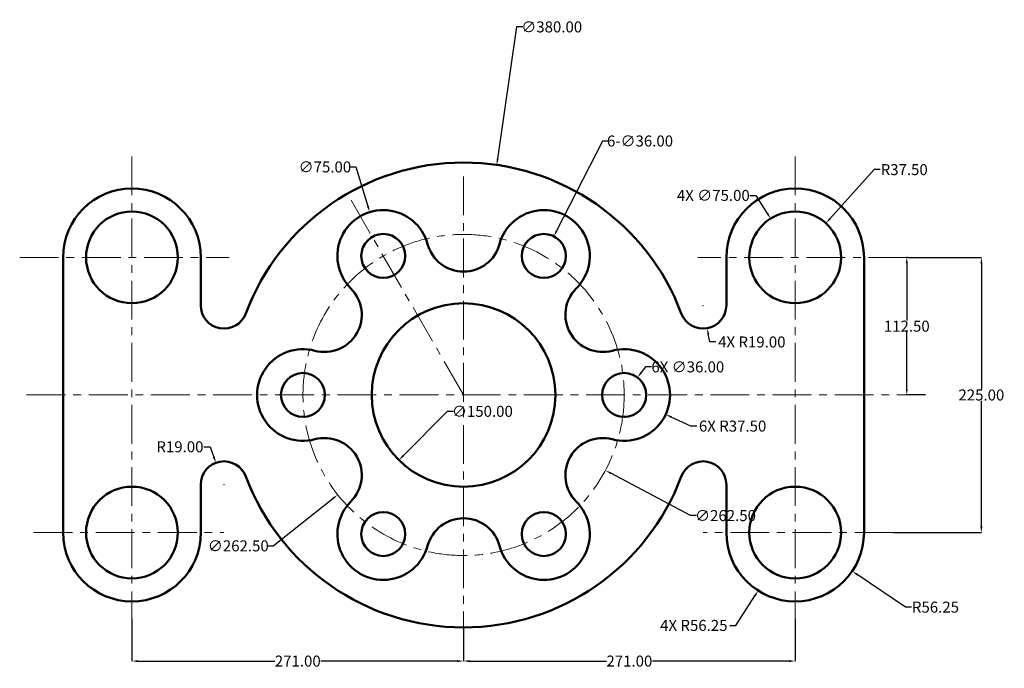
# Model space of a CAD drawing. Units: inches. Extents: x 559 to 1364, y 326 to 856.
import ezdxf

# ---------------------------------------------------------------- set-up
doc = ezdxf.new("R2010")
doc.units = ezdxf.units.IN
doc.header["$MEASUREMENT"] = 0
doc.linetypes.add('CENTER', pattern=[50.8, 31.75, -6.35, 6.35, -6.35])
for name, color, linetype, lineweight in [('M-CNTR', 4, 'CENTER', 18), ('M-DIMS', 2, 'Continuous', 25), ('M-OUTL', 7, 'Continuous', 50)]:
    doc.layers.add(name, color=color, linetype=linetype, lineweight=lineweight)
doc.styles.get("Standard").update_dxf_attribs({"font": 'arial.ttf'})
doc.dimstyles.get("Standard").update_dxf_attribs({"dimtxt": 9, "dimasz": 5, "dimexe": 0.18, "dimexo": 0.0625, "dimgap": 0.09, "dimtad": 0, "dimtih": 1, "dimtoh": 1, "dimzin": 0, "dimdsep": 46, "dimtxsty": 'Standard', "dimcen": 0.09, "dimadec": 0, "dimazin": 0, "dimtfac": 1, "dimtofl": 0, "dimtmove": 0, "dimatfit": 3, "dimfxl": 1, "dimtolj": 1, "dimtzin": 0, "dimarcsym": 0})

# ---------------------------------------------------------------- blocks, each defined once
blk = doc.blocks.new('*U1')
blk.add_arc((0, 19.16), 30.44, 195, 345)
blk = doc.blocks.new('*U2')
at = {"layer": 'M-OUTL', "color": 0, "linetype": 'ByBlock', "lineweight": -2, "transparency": 16777216}
blk.add_blockref('*U1', (921.89, 661.17), dxfattribs=at)
for p, rotation in [((824.82, 605.12), 59.99999999999999), ((1018.96, 605.12), 300), ((824.82, 493.03), 120), ((1018.96, 493.03), 240), ((921.89, 436.99), 180)]:
    blk.add_blockref('*U1', p, dxfattribs=dict(at, rotation=rotation))
blk = doc.blocks.new('*D3')
at = {"layer": 'Defpoints', "color": 0, "transparency": 16777216}
for p in [(1192.89, 436.58), (1239.47, 405.05)]:
    blk.add_point(p, dxfattribs=at)
at = {"layer": 'M-DIMS', "color": 0, "lineweight": -2, "transparency": 16777216}
for p, q in [((1192.8, 436.58), (1192.98, 436.58)), ((1192.89, 436.49), (1192.89, 436.67)), ((1282.92, 375.65), (1243.61, 402.25)), ((1287.92, 375.65), (1282.92, 375.65))]:
    blk.add_line(p, q, dxfattribs=at)
at = {"layer": 'M-DIMS', "color": 0, "transparency": 16777216}
blk.add_solid([(1244.08, 402.94), (1243.15, 401.56), (1239.47, 405.05)], dxfattribs=at)
at = {"layer": 'M-DIMS', "color": 0, "transparency": 16777216, "insert": (1307.53, 375.65), "char_height": 9, "attachment_point": 5}
blk.add_mtext('\\A1;R56.25', dxfattribs=at)
blk = doc.blocks.new('*D4')
at = {"layer": 'Defpoints', "color": 0, "transparency": 16777216}
for p in [(1217.97, 689.45), (1192.89, 661.58)]:
    blk.add_point(p, dxfattribs=at)
at = {"layer": 'M-DIMS', "color": 0, "lineweight": -2, "transparency": 16777216}
for p, q in [((1257.43, 733.3), (1221.32, 693.17)), ((1262.43, 733.3), (1257.43, 733.3)), ((1192.8, 661.58), (1192.98, 661.58)), ((1192.89, 661.49), (1192.89, 661.67))]:
    blk.add_line(p, q, dxfattribs=at)
at = {"layer": 'M-DIMS', "color": 0, "transparency": 16777216}
blk.add_solid([(1220.7, 693.73), (1221.94, 692.61), (1217.97, 689.45)], dxfattribs=at)
at = {"layer": 'M-DIMS', "color": 0, "transparency": 16777216, "insert": (1281.99, 733.3), "char_height": 9, "attachment_point": 5}
blk.add_mtext('\\A1;R37.50', dxfattribs=at)
blk = doc.blocks.new('*D5')
at = {"layer": 'Defpoints', "color": 0, "transparency": 16777216}
for p in [(1284.63, 661.58), (1284.07, 549.08), (1299.44, 549.08)]:
    blk.add_point(p, dxfattribs=at)
at = {"layer": 'M-DIMS', "color": 0, "lineweight": -2, "transparency": 16777216}
for p, q in [((1284.57, 661.58), (1283.89, 661.58)), ((1284.07, 656.58), (1284.07, 610.01)), ((1284.07, 554.08), (1284.07, 600.64)), ((1299.38, 549.08), (1283.89, 549.08))]:
    blk.add_line(p, q, dxfattribs=at)
at = {"layer": 'M-DIMS', "color": 0, "transparency": 16777216}
for points in [[(1283.24, 656.58), (1284.91, 656.58), (1284.07, 661.58)], [(1283.24, 554.08), (1284.91, 554.08), (1284.07, 549.08)]]:
    blk.add_solid(points, dxfattribs=at)
at = {"layer": 'M-DIMS', "color": 0, "transparency": 16777216, "insert": (1284.07, 605.33), "char_height": 9, "attachment_point": 5}
blk.add_mtext('\\A1;112.50', dxfattribs=at)
blk = doc.blocks.new('*D6')
at = {"layer": 'Defpoints', "color": 0, "transparency": 16777216}
for p in [(1284.63, 661.58), (1273.28, 436.58), (1345.05, 436.58)]:
    blk.add_point(p, dxfattribs=at)
at = {"layer": 'M-DIMS', "color": 0, "lineweight": -2, "transparency": 16777216}
for p, q in [((1284.7, 661.58), (1345.23, 661.58)), ((1345.05, 656.58), (1345.05, 553.76)), ((1345.05, 441.58), (1345.05, 544.39)), ((1273.34, 436.58), (1345.23, 436.58))]:
    blk.add_line(p, q, dxfattribs=at)
at = {"layer": 'M-DIMS', "color": 0, "transparency": 16777216}
for points in [[(1344.21, 656.58), (1345.88, 656.58), (1345.05, 661.58)], [(1344.21, 441.58), (1345.88, 441.58), (1345.05, 436.58)]]:
    blk.add_solid(points, dxfattribs=at)
at = {"layer": 'M-DIMS', "color": 0, "transparency": 16777216, "insert": (1345.05, 549.08), "char_height": 9, "attachment_point": 5}
blk.add_mtext('\\A1;225.00', dxfattribs=at)
blk = doc.blocks.new('*D7')
at = {"layer": 'Defpoints', "color": 0, "transparency": 16777216}
for p in [(995.68, 678.79), (979.35, 646.7)]:
    blk.add_point(p, dxfattribs=at)
at = {"layer": 'M-DIMS', "color": 0, "lineweight": -2, "transparency": 16777216}
for p, q in [((1035.31, 756.7), (997.94, 683.24)), ((1040.31, 756.7), (1035.31, 756.7)), ((987.42, 662.74), (987.6, 662.74)), ((987.51, 662.65), (987.51, 662.83))]:
    blk.add_line(p, q, dxfattribs=at)
at = {"layer": 'M-DIMS', "color": 0, "transparency": 16777216}
blk.add_solid([(997.2, 683.62), (998.69, 682.87), (995.68, 678.79)], dxfattribs=at)
at = {"layer": 'M-DIMS', "color": 0, "transparency": 16777216, "insert": (1066.08, 756.7), "char_height": 9, "attachment_point": 5}
blk.add_mtext('\\A1;6-∅36.00', dxfattribs=at)
blk = doc.blocks.new('*D8')
at = {"layer": 'Defpoints', "color": 0, "transparency": 16777216}
for p in [(845.17, 698.56), (867.36, 626.92)]:
    blk.add_point(p, dxfattribs=at)
at = {"layer": 'M-DIMS', "color": 0, "lineweight": -2, "transparency": 16777216}
for p, q in [((828.72, 735.51), (833.72, 735.51)), ((833.72, 735.51), (843.69, 703.34)), ((856.17, 662.74), (856.35, 662.74)), ((856.26, 662.65), (856.26, 662.83))]:
    blk.add_line(p, q, dxfattribs=at)
at = {"layer": 'M-DIMS', "color": 0, "transparency": 16777216}
blk.add_solid([(844.48, 703.59), (842.89, 703.09), (845.17, 698.56)], dxfattribs=at)
at = {"layer": 'M-DIMS', "color": 0, "transparency": 16777216, "insert": (808.56, 735.51), "char_height": 9, "attachment_point": 5}
blk.add_mtext('\\A1;∅75.00', dxfattribs=at)
blk = doc.blocks.new('*D9')
at = {"layer": 'Defpoints', "color": 0, "transparency": 16777216}
for p in [(719.52, 493.66), (726.14, 475.85)]:
    blk.add_point(p, dxfattribs=at)
at = {"layer": 'M-DIMS', "color": 0, "lineweight": -2, "transparency": 16777216}
for p, q in [((709.67, 506.73), (714.67, 506.73)), ((714.67, 506.73), (717.78, 498.34)), ((726.05, 475.85), (726.23, 475.85)), ((726.14, 475.76), (726.14, 475.94))]:
    blk.add_line(p, q, dxfattribs=at)
at = {"layer": 'M-DIMS', "color": 0, "transparency": 16777216}
blk.add_solid([(718.56, 498.63), (717, 498.05), (719.52, 493.66)], dxfattribs=at)
at = {"layer": 'M-DIMS', "color": 0, "transparency": 16777216, "insert": (690.1, 506.73), "char_height": 9, "attachment_point": 5}
blk.add_mtext('\\A1;R19.00', dxfattribs=at)
blk = doc.blocks.new('*D10')
at = {"layer": 'Defpoints', "color": 0, "transparency": 16777216}
for p in [(1024.71, 630.65), (819.07, 467.5)]:
    blk.add_point(p, dxfattribs=at)
at = {"layer": 'M-DIMS', "color": 0, "lineweight": -2, "transparency": 16777216}
for p, q in [((921.8, 549.08), (921.98, 549.08)), ((921.89, 548.99), (921.89, 549.17)), ((766.42, 425.74), (815.15, 464.4)), ((761.42, 425.74), (766.42, 425.74))]:
    blk.add_line(p, q, dxfattribs=at)
at = {"layer": 'M-DIMS', "color": 0, "transparency": 16777216}
blk.add_solid([(814.63, 465.05), (815.67, 463.74), (819.07, 467.5)], dxfattribs=at)
at = {"layer": 'M-DIMS', "color": 0, "transparency": 16777216, "insert": (737.77, 425.74), "char_height": 9, "attachment_point": 5}
blk.add_mtext('\\A1;∅262.50', dxfattribs=at)
blk = doc.blocks.new('*D11')
at = {"layer": 'Defpoints', "color": 0, "transparency": 16777216}
for p in [(650.89, 366.21), (921.89, 359.08), (921.89, 331.54)]:
    blk.add_point(p, dxfattribs=at)
at = {"layer": 'M-DIMS', "color": 0, "lineweight": -2, "transparency": 16777216}
for p, q in [((650.89, 366.15), (650.89, 331.36)), ((921.89, 359.02), (921.89, 331.36)), ((655.89, 331.54), (767.56, 331.54)), ((916.89, 331.54), (805.22, 331.54))]:
    blk.add_line(p, q, dxfattribs=at)
at = {"layer": 'M-DIMS', "color": 0, "transparency": 16777216}
for points in [[(655.89, 332.37), (655.89, 330.71), (650.89, 331.54)], [(916.89, 332.37), (916.89, 330.71), (921.89, 331.54)]]:
    blk.add_solid(points, dxfattribs=at)
at = {"layer": 'M-DIMS', "color": 0, "transparency": 16777216, "insert": (786.39, 331.54), "char_height": 9, "attachment_point": 5}
blk.add_mtext('\\A1;271.00', dxfattribs=at)
blk = doc.blocks.new('*D12')
at = {"layer": 'Defpoints', "color": 0, "transparency": 16777216}
for p in [(1192.89, 366.21), (921.89, 359.08), (1192.89, 331.54)]:
    blk.add_point(p, dxfattribs=at)
at = {"layer": 'M-DIMS', "color": 0, "lineweight": -2, "transparency": 16777216}
for p, q in [((1192.89, 366.15), (1192.89, 331.36)), ((921.89, 359.02), (921.89, 331.36)), ((926.89, 331.54), (1038.56, 331.54)), ((1187.89, 331.54), (1076.22, 331.54))]:
    blk.add_line(p, q, dxfattribs=at)
at = {"layer": 'M-DIMS', "color": 0, "transparency": 16777216}
for points in [[(926.89, 332.37), (926.89, 330.71), (921.89, 331.54)], [(1187.89, 332.37), (1187.89, 330.71), (1192.89, 331.54)]]:
    blk.add_solid(points, dxfattribs=at)
at = {"layer": 'M-DIMS', "color": 0, "transparency": 16777216, "insert": (1057.39, 331.54), "char_height": 9, "attachment_point": 5}
blk.add_mtext('\\A1;271.00', dxfattribs=at)
blk = doc.blocks.new('*D13')
at = {"layer": 'Defpoints', "color": 0, "transparency": 16777216}
for p in [(974.73, 602.3), (869.04, 495.86)]:
    blk.add_point(p, dxfattribs=at)
at = {"layer": 'M-DIMS', "color": 0, "lineweight": -2, "transparency": 16777216}
for p, q in [((908.6, 535.7), (872.57, 499.41)), ((913.6, 535.7), (908.6, 535.7))]:
    blk.add_line(p, q, dxfattribs=at)
at = {"layer": 'M-DIMS', "color": 0, "transparency": 16777216}
blk.add_solid([(871.97, 499.99), (873.16, 498.82), (869.04, 495.86)], dxfattribs=at)
at = {"layer": 'M-DIMS', "color": 0, "transparency": 16777216, "insert": (937.25, 535.7), "char_height": 9, "attachment_point": 5}
blk.add_mtext('\\A1;∅150.00', dxfattribs=at)
blk = doc.blocks.new('MOUNTING-EAR-D75')
blk.add_circle((0, 0), 37.5)
blk.add_arc((0, 0), 56.25, 180, 0)
blk = doc.blocks.new('HUB-LUG-D36')
blk.add_circle((0, 0), 18)
blk.add_arc((0, 0), 37.5, 75, 285)
blk = doc.blocks.new('*D16')
at = {"layer": 'Defpoints', "color": 0, "transparency": 16777216}
for p in [(949, 737.13), (894.78, 361.02)]:
    blk.add_point(p, dxfattribs=at)
at = {"layer": 'M-DIMS', "color": 0, "lineweight": -2, "transparency": 16777216}
for p, q in [((965.27, 849.97), (949.71, 742.08)), ((970.27, 849.97), (965.27, 849.97)), ((921.8, 549.08), (921.98, 549.08)), ((921.89, 548.99), (921.89, 549.17))]:
    blk.add_line(p, q, dxfattribs=at)
at = {"layer": 'M-DIMS', "color": 0, "transparency": 16777216}
blk.add_solid([(948.89, 742.2), (950.54, 741.96), (949, 737.13)], dxfattribs=at)
at = {"layer": 'M-DIMS', "color": 0, "transparency": 16777216, "insert": (993.92, 849.97), "char_height": 9, "attachment_point": 5}
blk.add_mtext('\\A1;∅380.00', dxfattribs=at)
blk = doc.blocks.new('*D17')
at = {"layer": 'Defpoints', "color": 0, "transparency": 16777216}
for p in [(1172.8, 693.24), (1212.98, 629.91)]:
    blk.add_point(p, dxfattribs=at)
at = {"layer": 'M-DIMS', "color": 0, "lineweight": -2, "transparency": 16777216}
for p, q in [((1155.74, 712.24), (1160.74, 712.24)), ((1160.74, 712.24), (1170.12, 697.46)), ((1192.8, 661.58), (1192.98, 661.58)), ((1192.89, 661.49), (1192.89, 661.67))]:
    blk.add_line(p, q, dxfattribs=at)
at = {"layer": 'M-DIMS', "color": 0, "transparency": 16777216}
blk.add_solid([(1170.82, 697.91), (1169.42, 697.02), (1172.8, 693.24)], dxfattribs=at)
at = {"layer": 'M-DIMS', "color": 0, "transparency": 16777216, "insert": (1125.98, 712.24), "char_height": 9, "attachment_point": 5}
blk.add_mtext('\\A1;4X ∅75.00', dxfattribs=at)
blk = doc.blocks.new('*D18')
at = {"layer": 'Defpoints', "color": 0, "transparency": 16777216}
for p in [(1192.89, 436.58), (1162.65, 389.15)]:
    blk.add_point(p, dxfattribs=at)
at = {"layer": 'M-DIMS', "color": 0, "lineweight": -2, "transparency": 16777216}
for p, q in [((1192.8, 436.58), (1192.98, 436.58)), ((1192.89, 436.49), (1192.89, 436.67)), ((1144.5, 360.69), (1159.96, 384.93)), ((1139.5, 360.69), (1144.5, 360.69))]:
    blk.add_line(p, q, dxfattribs=at)
at = {"layer": 'M-DIMS', "color": 0, "transparency": 16777216}
blk.add_solid([(1159.26, 385.38), (1160.66, 384.48), (1162.65, 389.15)], dxfattribs=at)
at = {"layer": 'M-DIMS', "color": 0, "transparency": 16777216, "insert": (1110.04, 360.69), "char_height": 9, "attachment_point": 5}
blk.add_mtext('\\A1;4X R56.25', dxfattribs=at)
blk = doc.blocks.new('*D19')
at = {"layer": 'Defpoints', "color": 0, "transparency": 16777216}
for p in [(1117.64, 622.31), (1121.02, 603.61)]:
    blk.add_point(p, dxfattribs=at)
at = {"layer": 'M-DIMS', "color": 0, "lineweight": -2, "transparency": 16777216}
for p, q in [((1117.55, 622.31), (1117.73, 622.31)), ((1117.64, 622.22), (1117.64, 622.4)), ((1123.05, 592.4), (1121.91, 598.69)), ((1128.05, 592.4), (1123.05, 592.4))]:
    blk.add_line(p, q, dxfattribs=at)
at = {"layer": 'M-DIMS', "color": 0, "transparency": 16777216}
blk.add_solid([(1122.73, 598.84), (1121.09, 598.54), (1121.02, 603.61)], dxfattribs=at)
at = {"layer": 'M-DIMS', "color": 0, "transparency": 16777216, "insert": (1157.46, 592.4), "char_height": 9, "attachment_point": 5}
blk.add_mtext('\\A1;4X R19.00', dxfattribs=at)
blk = doc.blocks.new('*D20')
at = {"layer": 'Defpoints', "color": 0, "transparency": 16777216}
for p in [(1053.14, 549.08), (1087.11, 533.19)]:
    blk.add_point(p, dxfattribs=at)
at = {"layer": 'M-DIMS', "color": 0, "lineweight": -2, "transparency": 16777216}
for p, q in [((1053.05, 549.08), (1053.23, 549.08)), ((1053.14, 548.99), (1053.14, 549.17)), ((1107.49, 523.65), (1091.63, 531.07)), ((1112.49, 523.65), (1107.49, 523.65))]:
    blk.add_line(p, q, dxfattribs=at)
at = {"layer": 'M-DIMS', "color": 0, "transparency": 16777216}
blk.add_solid([(1091.99, 531.82), (1091.28, 530.31), (1087.11, 533.19)], dxfattribs=at)
at = {"layer": 'M-DIMS', "color": 0, "transparency": 16777216, "insert": (1141.75, 523.65), "char_height": 9, "attachment_point": 5}
blk.add_mtext('\\A1;6X R37.50', dxfattribs=at)
blk = doc.blocks.new('*D21')
at = {"layer": 'Defpoints', "color": 0, "transparency": 16777216}
for p in [(1064.02, 563.42), (1042.26, 534.74)]:
    blk.add_point(p, dxfattribs=at)
at = {"layer": 'M-DIMS', "color": 0, "lineweight": -2, "transparency": 16777216}
for p, q in [((1070.54, 572.03), (1067.04, 567.4)), ((1075.54, 572.03), (1070.54, 572.03)), ((1053.05, 549.08), (1053.23, 549.08)), ((1053.14, 548.99), (1053.14, 549.17))]:
    blk.add_line(p, q, dxfattribs=at)
at = {"layer": 'M-DIMS', "color": 0, "transparency": 16777216}
blk.add_solid([(1066.37, 567.91), (1067.7, 566.9), (1064.02, 563.42)], dxfattribs=at)
at = {"layer": 'M-DIMS', "color": 0, "transparency": 16777216, "insert": (1105.15, 572.03), "char_height": 9, "attachment_point": 5}
blk.add_mtext('\\A1;6X ∅36.00', dxfattribs=at)
blk = doc.blocks.new('*D22')
at = {"layer": 'Defpoints', "color": 0, "transparency": 16777216}
for p in [(806, 610.7), (1037.77, 487.46)]:
    blk.add_point(p, dxfattribs=at)
at = {"layer": 'M-DIMS', "color": 0, "lineweight": -2, "transparency": 16777216}
for p, q in [((921.8, 549.08), (921.98, 549.08)), ((921.89, 548.99), (921.89, 549.17)), ((1107.31, 450.49), (1042.19, 485.11)), ((1112.31, 450.49), (1107.31, 450.49))]:
    blk.add_line(p, q, dxfattribs=at)
at = {"layer": 'M-DIMS', "color": 0, "transparency": 16777216}
blk.add_solid([(1042.58, 485.85), (1041.8, 484.37), (1037.77, 487.46)], dxfattribs=at)
at = {"layer": 'M-DIMS', "color": 0, "transparency": 16777216, "insert": (1135.96, 450.49), "char_height": 9, "attachment_point": 5}
blk.add_mtext('\\A1;∅262.50', dxfattribs=at)

msp = doc.modelspace()

# ---------------------------------------------------------------- linework, layer by layer
at = {"layer": 'M-CNTR'}
for p, q in [((650.889, 744.109), (650.889, 366.21)), ((1192.889, 744.109), (1192.889, 366.21)), ((921.889, 727.694), (921.889, 359.078)), ((921.889, 549.078), (830.016, 708.207)), ((559.143, 661.578), (730.4, 661.578)), ((1284.634, 661.578), (1113.377, 661.578)), ((564.837, 549.078), (1299.438, 549.078)), ((570.502, 436.578), (726.031, 436.578)), ((1273.275, 436.578), (1117.746, 436.578))]:
    msp.add_line(p, q, dxfattribs=at)
msp.add_circle((921.889, 549.078), 131.25, dxfattribs=at)
at = {"layer": 'M-OUTL'}
for p, q in [((594.639, 436.578), (594.639, 661.578)), ((707.139, 622.31), (707.139, 661.578)), ((1136.639, 622.31), (1136.639, 661.578)), ((1249.139, 436.578), (1249.139, 661.578)), ((707.139, 436.578), (707.139, 475.846)), ((1136.639, 436.578), (1136.639, 475.846))]:
    msp.add_line(p, q, dxfattribs=at)
for centre, radius in [((921.889, 549.078), 75), ((790.639, 549.078), 18), ((1053.139, 549.078), 18)]:
    msp.add_circle(centre, radius, dxfattribs=at)
for centre, radius, start, end in [((921.889, 549.078), 190, 20.511338, 159.488662), ((726.139, 622.31), 19, 180, 339.488662), ((1117.639, 622.31), 19, 200.511338, 0), ((726.139, 475.846), 19, 20.511338, 180), ((1117.639, 475.846), 19, 0, 159.488662), ((921.889, 549.078), 190, 200.511338, 339.488662)]:
    msp.add_arc(centre, radius, start, end, dxfattribs=at)

# ---------------------------------------------------------------- block references
for name, p, rotation in [('MOUNTING-EAR-D75', (650.889, 661.578), 180), ('MOUNTING-EAR-D75', (1192.889, 661.578), 180), ('HUB-LUG-D36', (856.264, 662.744), 300.0000002742606), ('HUB-LUG-D36', (987.514, 662.744), 239.9999997257399), ('HUB-LUG-D36', (1053.139, 549.078), 180), ('HUB-LUG-D36', (856.264, 435.412), 59.99999972573956), ('HUB-LUG-D36', (987.514, 435.412), 120.0000002742606)]:
    msp.add_blockref(name, p, dxfattribs=dict(at, rotation=rotation))
for name, p in [('*U2', (0, 0)), ('HUB-LUG-D36', (790.639, 549.078)), ('MOUNTING-EAR-D75', (650.889, 436.578)), ('MOUNTING-EAR-D75', (1192.889, 436.578))]:
    msp.add_blockref(name, p, dxfattribs=at)

# ---------------------------------------------------------------- dimensions: what is measured, and where the dimension line sits
at = {"layer": 'M-DIMS'}
for p1, p2, override, picture, middle in [((894.777, 361.022), (949.001, 737.133), {"dimdec": 2, "dimlfac": 1, "dimrnd": 0, "dimzin": 0, "dimdsep": 46, "dimlunit": 2}, '*D16', (993.92, 849.967)), ((867.361, 626.923), (845.166, 698.564), {"dimclrd": 0, "dimclre": 0, "dimclrt": 0}, '*D8', (808.565, 735.508)), ((1024.71, 630.651), (819.067, 467.504), {"dimclrd": 0, "dimclre": 0, "dimclrt": 0}, '*D10', (737.77, 425.738)), ((806.003, 610.698), (1037.774, 487.458), {"dimdec": 2, "dimlfac": 1, "dimrnd": 0, "dimzin": 0, "dimdsep": 46, "dimlunit": 2}, '*D22', (1135.958, 450.486)), ((974.735, 602.297), (869.042, 495.859), {"dimclrd": 0, "dimclre": 0, "dimclrt": 0}, '*D13', (937.254, 535.697))]:
    dim = msp.add_diameter_dim_2p(p1=p1, p2=p2, dimstyle='Standard', override=override, dxfattribs=at)
    dim.commit()
    dim.dimension.update_dxf_attribs({"geometry": picture, "text_midpoint": middle, "dimtype": 163})
for p1, p2, text, override, picture, middle in [((979.352, 646.7), (995.675, 678.787), '6-<>', {"dimclrd": 0, "dimclre": 0, "dimclrt": 0}, '*D7', (1066.075, 756.699)), ((1212.979, 629.913), (1172.799, 693.242), '4X <>', {"dimdec": 2, "dimlfac": 1, "dimrnd": 0, "dimzin": 0, "dimdsep": 46, "dimlunit": 2}, '*D17', (1125.978, 712.241)), ((1042.262, 534.736), (1064.015, 563.42), '6X <>', {"dimdec": 2, "dimlfac": 1, "dimrnd": 0, "dimzin": 0, "dimdsep": 46, "dimlunit": 2}, '*D21', (1105.151, 572.025))]:
    dim = msp.add_diameter_dim_2p(p1=p1, p2=p2, text=text, dimstyle='Standard', override=override, dxfattribs=at)
    dim.commit()
    dim.dimension.update_dxf_attribs({"geometry": picture, "text_midpoint": middle, "dimtype": 163})
for center, mpoint, picture, middle in [((1192.889, 661.578), (1217.973, 689.453), '*D4', (1281.994, 733.299)), ((726.139, 475.846), (719.523, 493.657), '*D9', (690.101, 506.729)), ((1192.889, 436.578), (1239.473, 405.05), '*D3', (1307.533, 375.648))]:
    dim = msp.add_radius_dim(center=center, mpoint=mpoint, dimstyle='Standard', override={"dimclrd": 0, "dimclre": 0, "dimclrt": 0}, dxfattribs=at)
    dim.commit()
    dim.dimension.update_dxf_attribs({"geometry": picture, "text_midpoint": middle, "dimtype": 164})
for base, p2, picture, middle in [((1284.073, 549.078), (1299.438, 549.078), '*D5', (1284.073, 605.328)), ((1345.045, 436.578), (1273.275, 436.578), '*D6', (1345.045, 549.078))]:
    dim = msp.add_linear_dim(base=base, p1=(1284.634, 661.578), p2=p2, angle=90, dimstyle='Standard', override={"dimclrd": 0, "dimclre": 0, "dimclrt": 0}, dxfattribs=at)
    dim.commit()
    dim.dimension.update_dxf_attribs({"geometry": picture, "text_midpoint": middle})
for center, mpoint, text, picture, middle in [((1117.639, 622.31), (1121.019, 603.613), '4X <>', '*D19', (1157.465, 592.395)), ((1053.139, 549.078), (1087.105, 533.187), '6X <>', '*D20', (1141.745, 523.652)), ((1192.889, 436.578), (1162.649, 389.148), '4X <>', '*D18', (1110.039, 360.69))]:
    dim = msp.add_radius_dim(center=center, mpoint=mpoint, text=text, dimstyle='Standard', override={"dimdec": 2, "dimlfac": 1, "dimrnd": 0, "dimzin": 0, "dimdsep": 46, "dimlunit": 2}, dxfattribs=at)
    dim.commit()
    dim.dimension.update_dxf_attribs({"geometry": picture, "text_midpoint": middle, "dimtype": 164})
for base, p1, p2, picture, middle in [((921.889, 331.54), (650.889, 366.21), (921.889, 359.078), '*D11', (786.389, 331.54)), ((1192.889, 331.54), (921.889, 359.078), (1192.889, 366.21), '*D12', (1057.389, 331.54))]:
    dim = msp.add_linear_dim(base=base, p1=p1, p2=p2, dimstyle='Standard', override={"dimclrd": 0, "dimclre": 0, "dimclrt": 0}, dxfattribs=at)
    dim.commit()
    dim.dimension.update_dxf_attribs({"geometry": picture, "text_midpoint": middle})

doc.saveas('drawing.dxf')
